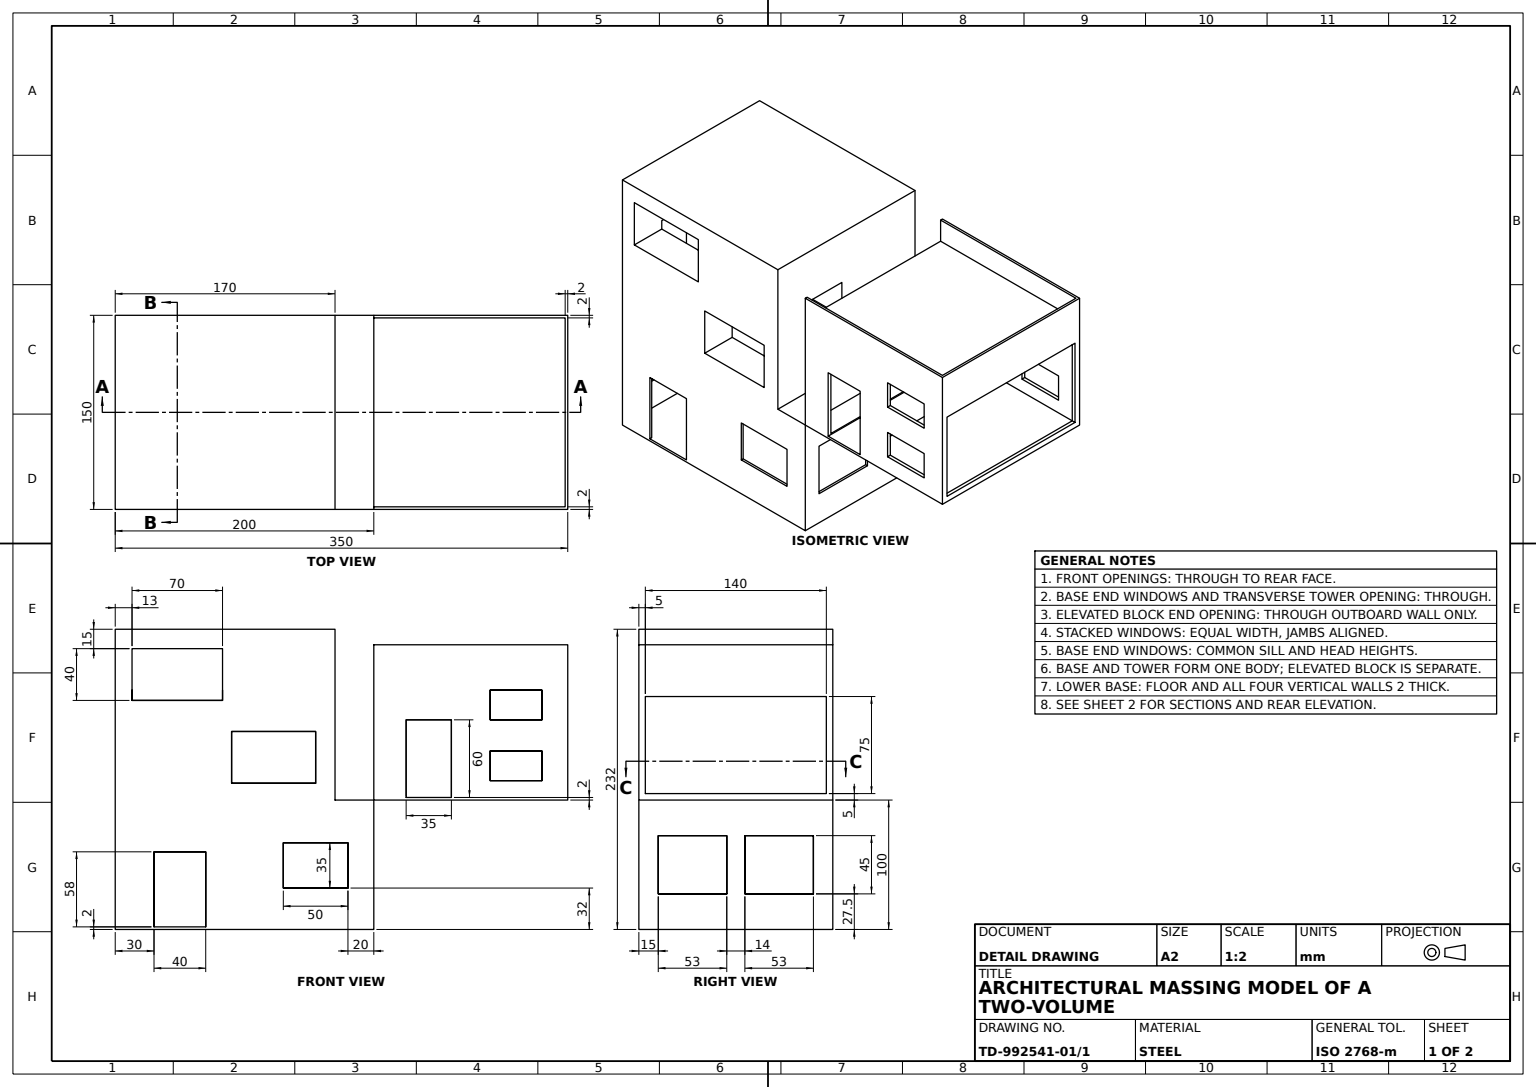
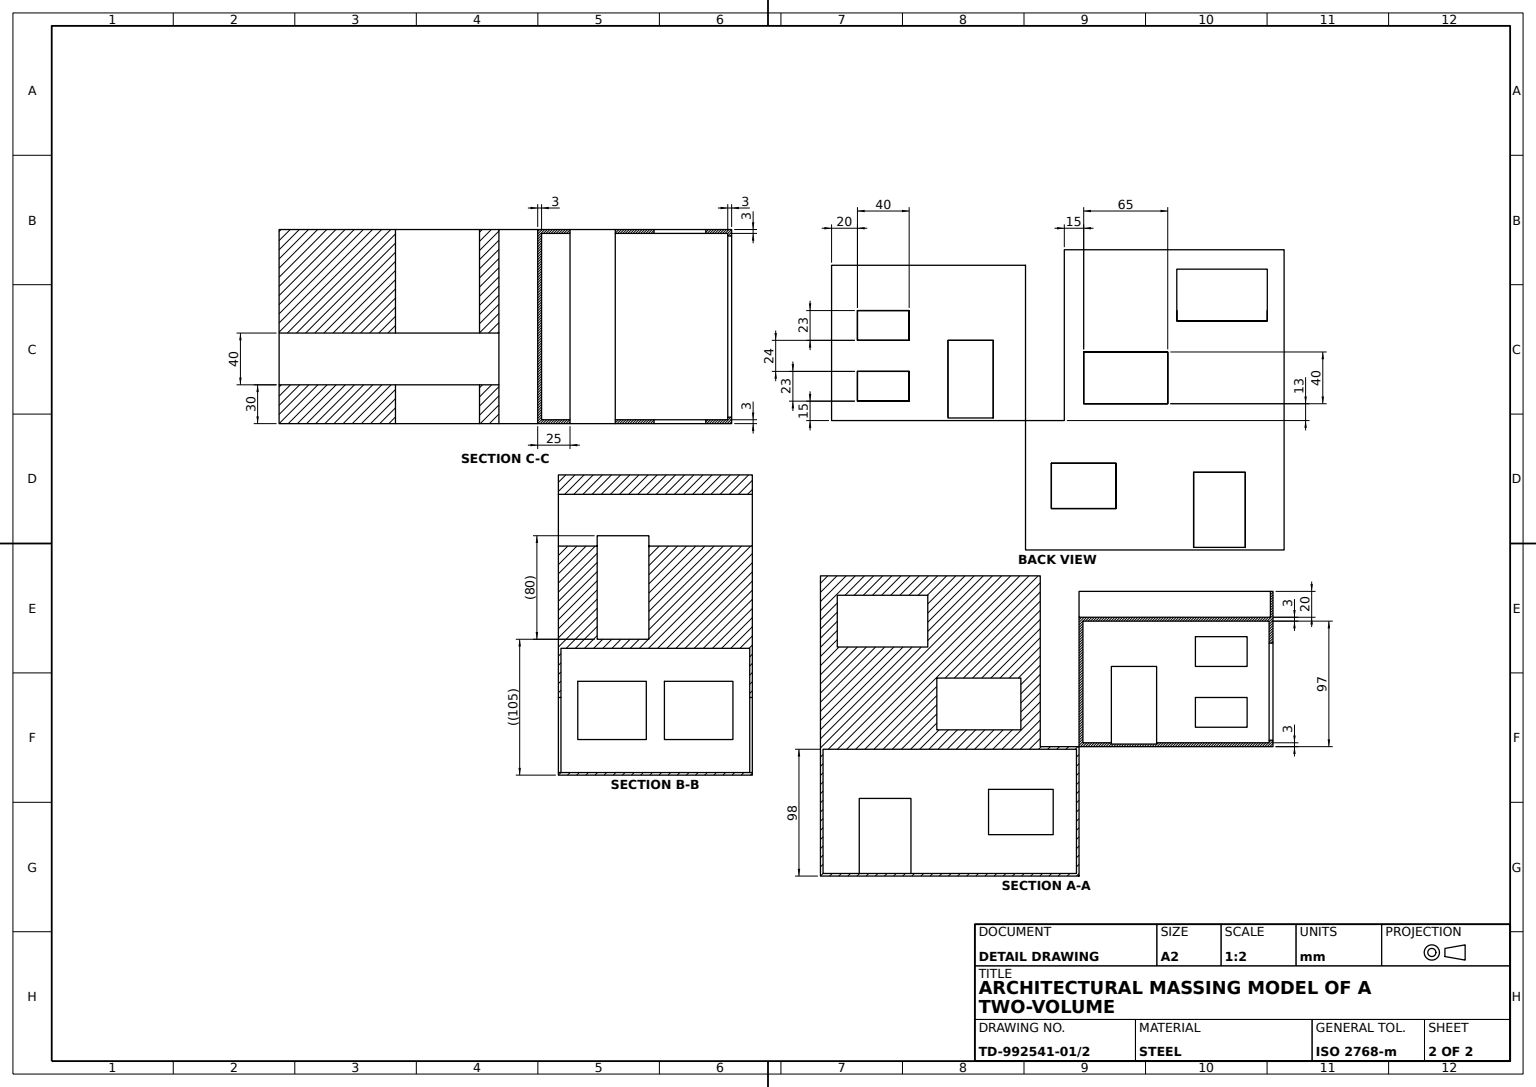
from build123d import *

# Parameters (mm, degrees)
BASE_BLOCK_SKETCH_W               = 200
BASE_BLOCK_SKETCH_H               = 150
BASE_BLOCK_DEPTH                  = 100
BASE_DOOR_OPENING_SKETCH_W        = 40
BASE_DOOR_OPENING_SKETCH_H        = 58
BASE_DOOR_OPENING_DEPTH           = 270
BASE_HOLLOW_SKETCH_W              = 196
BASE_HOLLOW_SKETCH_H              = 146
BASE_HOLLOW_2MM_WALL_DEPTH        = 98
BASE_FLOOR_SLAB_SKETCH_W          = 200
BASE_FLOOR_SLAB_SKETCH_H          = 150
BASE_FLOOR_SLAB_DEPTH             = 2
BASE_WINDOW_SKETCH_W              = 50
BASE_WINDOW_SKETCH_H              = 35
BASE_WINDOW_DEPTH                 = 332
BASE_SIDE_WINDOWS_SKETCH_W        = 53
BASE_SIDE_WINDOWS_SKETCH_H        = 45
BASE_SIDE_WINDOWS_DEPTH           = 332
SIDE_BLOCK_SKETCH_W               = 150
SIDE_BLOCK_SKETCH_H               = 150
SIDE_BLOCK_DEPTH                  = 100
SIDE_BLOCK_HOLLOW_SKETCH_W        = 144
SIDE_BLOCK_HOLLOW_SKETCH_H        = 144
SIDE_BLOCK_HOLLOW_3MM_WALL_DEPTH  = 97
SIDE_BLOCK_FLOOR_SLAB_SKETCH_W    = 150
SIDE_BLOCK_FLOOR_SLAB_SKETCH_H    = 150
SIDE_BLOCK_FLOOR_SLAB_DEPTH       = 3
SIDE_BLOCK_DOOR_SKETCH_W          = 35
SIDE_BLOCK_DOOR_SKETCH_H          = 60
SIDE_BLOCK_DOOR_OPENING_DEPTH     = 213
SIDE_BLOCK_WINDOWS_SKETCH_W       = 40
SIDE_BLOCK_WINDOWS_SKETCH_H       = 23
SIDE_BLOCK_WINDOWS_DEPTH          = 213
SIDE_BLOCK_FRONT_OPENING_SKETCH_W = 140
SIDE_BLOCK_FRONT_OPENING_SKETCH_H = 75
SIDE_BLOCK_FRONT_OPENING_DEPTH    = 113
PARAPET_FRONT_SKETCH_W            = 150
PARAPET_FRONT_SKETCH_H            = 20
PARAPET_FRONT_DEPTH               = 2
PARAPET_SIDE_SKETCH_W             = 147
PARAPET_SIDE_SKETCH_H             = 20
PARAPET_SIDE_DEPTH                = 2
PARAPET_BACK_SKETCH_W             = 150
PARAPET_BACK_SKETCH_H             = 20
PARAPET_BACK_DEPTH                = 2
TOWER_SKETCH_W                    = 170
TOWER_SKETCH_H                    = 150
TOWER_EXTENSION_DEPTH             = 132
TOWER_WINDOWS_SKETCH_W            = 65
TOWER_WINDOWS_SKETCH_H            = 40
TOWER_WINDOWS_SKETCH_W_2          = 70
TOWER_WINDOWS_DEPTH               = 152
TOWER_WINDOW_OPENING_SKETCH_W     = 40
TOWER_WINDOW_OPENING_SKETCH_H     = 80
TOWER_WINDOW_OPENING_DEPTH        = 206


with BuildPart() as part:
    # Base Block Sketch → Base Block (new body)
    with BuildSketch(Plane(origin=(0, 0, 0), x_dir=(1, 0, 0), z_dir=(0, 1, 0))):
        with Locations((100, 75)):
            Rectangle(BASE_BLOCK_SKETCH_W, BASE_BLOCK_SKETCH_H)
    extrude(amount=BASE_BLOCK_DEPTH)

    # Base Door Opening Sketch → Base Door Opening (cut)
    with BuildSketch(Plane.XY):
        with Locations((50, 31)):
            Rectangle(BASE_DOOR_OPENING_SKETCH_W, BASE_DOOR_OPENING_SKETCH_H)
    extrude(amount=-BASE_DOOR_OPENING_DEPTH, mode=Mode.SUBTRACT)

    # Base Hollow Sketch → Base Hollow 2mm Wall (cut)
    with BuildSketch(Plane(origin=(0, 100, 0), x_dir=(1, 0, 0), z_dir=(0, 1, 0))):
        with Locations((100, 75)):
            Rectangle(BASE_HOLLOW_SKETCH_W, BASE_HOLLOW_SKETCH_H)
    extrude(amount=-BASE_HOLLOW_2MM_WALL_DEPTH, mode=Mode.SUBTRACT)

    # Base Floor Slab Sketch → Base Floor Slab (add)
    with BuildSketch(Plane(origin=(0, 100, 0), x_dir=(1, 0, 0), z_dir=(0, 1, 0))):
        with Locations((100, 75)):
            Rectangle(BASE_FLOOR_SLAB_SKETCH_W, BASE_FLOOR_SLAB_SKETCH_H)
    extrude(amount=-BASE_FLOOR_SLAB_DEPTH)

    # Base Window Sketch → Base Window (cut)
    with BuildSketch(Plane.XY):
        with Locations((155, 49.5)):
            Rectangle(BASE_WINDOW_SKETCH_W, BASE_WINDOW_SKETCH_H)
    extrude(amount=-BASE_WINDOW_DEPTH, mode=Mode.SUBTRACT)

    # Base Side Windows Sketch → Base Side Windows (cut)
    with BuildSketch(Plane(origin=(200, 0, 0), x_dir=(0, 0, -1), z_dir=(1, 0, 0))):
        with Locations((41.5, 50)):
            Rectangle(BASE_SIDE_WINDOWS_SKETCH_W, BASE_SIDE_WINDOWS_SKETCH_H)
        with Locations((108.5, 50)):
            Rectangle(BASE_SIDE_WINDOWS_SKETCH_W, BASE_SIDE_WINDOWS_SKETCH_H)
    extrude(amount=-BASE_SIDE_WINDOWS_DEPTH, mode=Mode.SUBTRACT)

    # Tower Sketch → Tower Extension (add)
    with BuildSketch(Plane(origin=(0, 100, 0), x_dir=(1, 0, 0), z_dir=(0, 1, 0))):
        with Locations((85, 75)):
            Rectangle(TOWER_SKETCH_W, TOWER_SKETCH_H)
    extrude(amount=TOWER_EXTENSION_DEPTH)

    # Tower Windows Sketch → Tower Windows (cut)
    with BuildSketch(Plane.XY):
        with Locations((122.5, 133)):
            Rectangle(TOWER_WINDOWS_SKETCH_W, TOWER_WINDOWS_SKETCH_H)
        with Locations((48, 197)):
            Rectangle(TOWER_WINDOWS_SKETCH_W_2, TOWER_WINDOWS_SKETCH_H)
    extrude(amount=-TOWER_WINDOWS_DEPTH, mode=Mode.SUBTRACT)

    # Tower Window Opening Sketch → Tower Window Opening (cut)
    with BuildSketch(Plane(origin=(170, 0, 0), x_dir=(0, 0, -1), z_dir=(1, 0, 0))):
        with Locations((50, 145)):
            Rectangle(TOWER_WINDOW_OPENING_SKETCH_W, TOWER_WINDOW_OPENING_SKETCH_H)
    extrude(amount=-TOWER_WINDOW_OPENING_DEPTH, mode=Mode.SUBTRACT)


with BuildPart() as body_2:
    # Side Block Sketch → Side Block (new body)
    with BuildSketch(Plane(origin=(0, 100, 0), x_dir=(1, 0, 0), z_dir=(0, 1, 0))):
        with Locations((275, 75)):
            Rectangle(SIDE_BLOCK_SKETCH_W, SIDE_BLOCK_SKETCH_H)
    extrude(amount=SIDE_BLOCK_DEPTH)

    # Side Block Hollow Sketch → Side Block Hollow 3mm Wall (cut)
    with BuildSketch(Plane(origin=(0, 200, 0), x_dir=(1, 0, 0), z_dir=(0, 1, 0))):
        with Locations((275, 75)):
            Rectangle(SIDE_BLOCK_HOLLOW_SKETCH_W, SIDE_BLOCK_HOLLOW_SKETCH_H)
    extrude(amount=-SIDE_BLOCK_HOLLOW_3MM_WALL_DEPTH, mode=Mode.SUBTRACT)

    # Side Block Floor Slab Sketch → Side Block Floor Slab (add)
    with BuildSketch(Plane(origin=(0, 200, 0), x_dir=(1, 0, 0), z_dir=(0, 1, 0))):
        with Locations((275, 75)):
            Rectangle(SIDE_BLOCK_FLOOR_SLAB_SKETCH_W, SIDE_BLOCK_FLOOR_SLAB_SKETCH_H)
    extrude(amount=-SIDE_BLOCK_FLOOR_SLAB_DEPTH)

    # Side Block Door Sketch → Side Block Door Opening (cut)
    with BuildSketch(Plane.XY):
        with Locations((242.5, 132)):
            Rectangle(SIDE_BLOCK_DOOR_SKETCH_W, SIDE_BLOCK_DOOR_SKETCH_H)
    extrude(amount=-SIDE_BLOCK_DOOR_OPENING_DEPTH, mode=Mode.SUBTRACT)

    # Side Block Windows Sketch → Side Block Windows (cut)
    with BuildSketch(Plane.XY):
        with Locations((310, 126.5)):
            Rectangle(SIDE_BLOCK_WINDOWS_SKETCH_W, SIDE_BLOCK_WINDOWS_SKETCH_H)
        with Locations((310, 173.5)):
            Rectangle(SIDE_BLOCK_WINDOWS_SKETCH_W, SIDE_BLOCK_WINDOWS_SKETCH_H)
    extrude(amount=-SIDE_BLOCK_WINDOWS_DEPTH, mode=Mode.SUBTRACT)

    # Side Block Front Opening Sketch → Side Block Front Opening (cut)
    with BuildSketch(Plane(origin=(350, 0, 0), x_dir=(0, 0, -1), z_dir=(1, 0, 0))):
        with Locations((75, 142.5)):
            Rectangle(SIDE_BLOCK_FRONT_OPENING_SKETCH_W, SIDE_BLOCK_FRONT_OPENING_SKETCH_H)
    extrude(amount=-SIDE_BLOCK_FRONT_OPENING_DEPTH, mode=Mode.SUBTRACT)

    # Parapet Front Sketch → Parapet Front (add)
    with BuildSketch(Plane.XY):
        with Locations((275, 210)):
            Rectangle(PARAPET_FRONT_SKETCH_W, PARAPET_FRONT_SKETCH_H)
    extrude(amount=-PARAPET_FRONT_DEPTH)

    # Parapet Side Sketch → Parapet Side (add)
    with BuildSketch(Plane(origin=(350, 0, 0), x_dir=(0, 0, -1), z_dir=(1, 0, 0))):
        with Locations((75.5, 210)):
            Rectangle(PARAPET_SIDE_SKETCH_W, PARAPET_SIDE_SKETCH_H)
    extrude(amount=-PARAPET_SIDE_DEPTH)

    # Parapet Back Sketch → Parapet Back (add)
    with BuildSketch(Plane(origin=(0, 0, -150), x_dir=(-1, 0, 0), z_dir=(0, 0, -1))):
        with Locations((-275, 210)):
            Rectangle(PARAPET_BACK_SKETCH_W, PARAPET_BACK_SKETCH_H)
    extrude(amount=-PARAPET_BACK_DEPTH)


solid = Compound([part.part, body_2.part])
